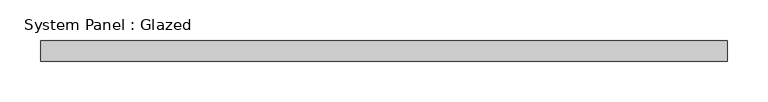
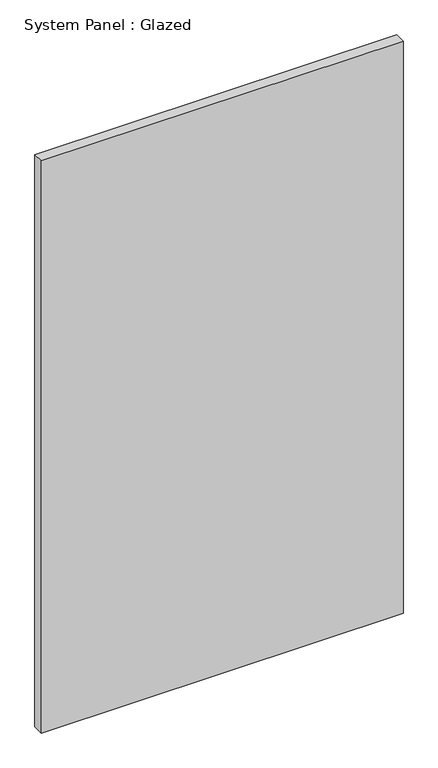
"""IFC4 building model written with IfcOpenShell, lengths in millimetres: plate geometry, System Panel : Glazed."""

from ifc_helpers import new_model, si_unit, origin, origin_with_axes, place, context, project, spatial, polyline, outline, extrude, source, transform, mapped, element, save


def system_panel_glazed_e9dc8a15(model_context):
    return source(origin(), model_context, "Body", "SweptSolid", [
        extrude(outline(polyline([(423.8625, 19.05), (-423.8625, 19.05), (-423.8625, 44.45), (423.8625, 44.45), (423.8625, 19.05)])), origin_with_axes(), (0.0, 0.0, 1.0), 1417.0388529),
    ])


if __name__ == "__main__":
    model = new_model("IFC4")
    model_context = context("Model", 3, world=origin())
    ifc_project = project(units=[si_unit("LENGTHUNIT", "METRE", prefix="MILLI")], contexts=[model_context])
    site = spatial("IfcSite", under=ifc_project)
    building = spatial("IfcBuilding", under=site)
    placement = place(None, origin())
    system_panel_glazed_shape = system_panel_glazed_e9dc8a15(model_context)
    element("IfcPlate", 1, ObjectType="System Panel : Glazed", at=placement, inside=building, context=model_context, shape_type="MappedRepresentation", body=[
        mapped(system_panel_glazed_shape, transform((0.0, 0.0, 0.0), x_axis=(1.0, 0.0, 0.0), y_axis=(0.0, 1.0, 0.0), z_axis=(0.0, 0.0, 1.0))),
    ])
    save(model, "model.ifc")

# Revit data of these elements
# Type "System Panel : Glazed"
#   Construction Type Id = "GSP4R"
#   Analytic Construction = "1/8 in Pilkington single glazing"
#   Visual Light Transmittance = 0.9
#   Solar Heat Gain Coefficient = 0.86
#   Heat Transfer Coefficient (U) = 1.18115 BTU/(h·ft²·°F)
#   Define Thermal Properties by = 1
# Element 1 (IfcPlate, "System Panel : Glazed")
#   Materials on its faces: "Glass"
# Materials
#   "Glass": class "Glass", colour RGB 0 128 192, transparency 0.75, Description = "Soda Lime Glass", Cost = 0
